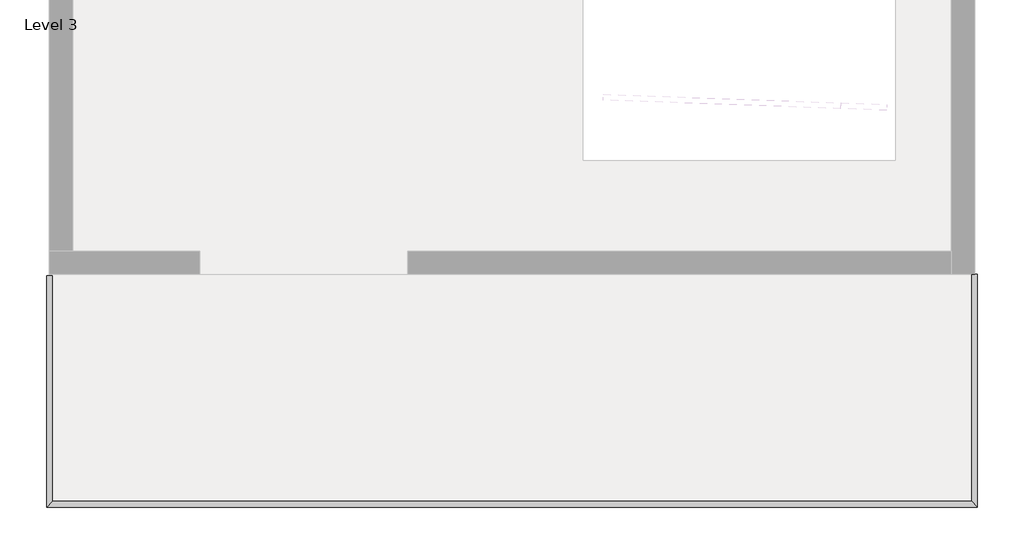
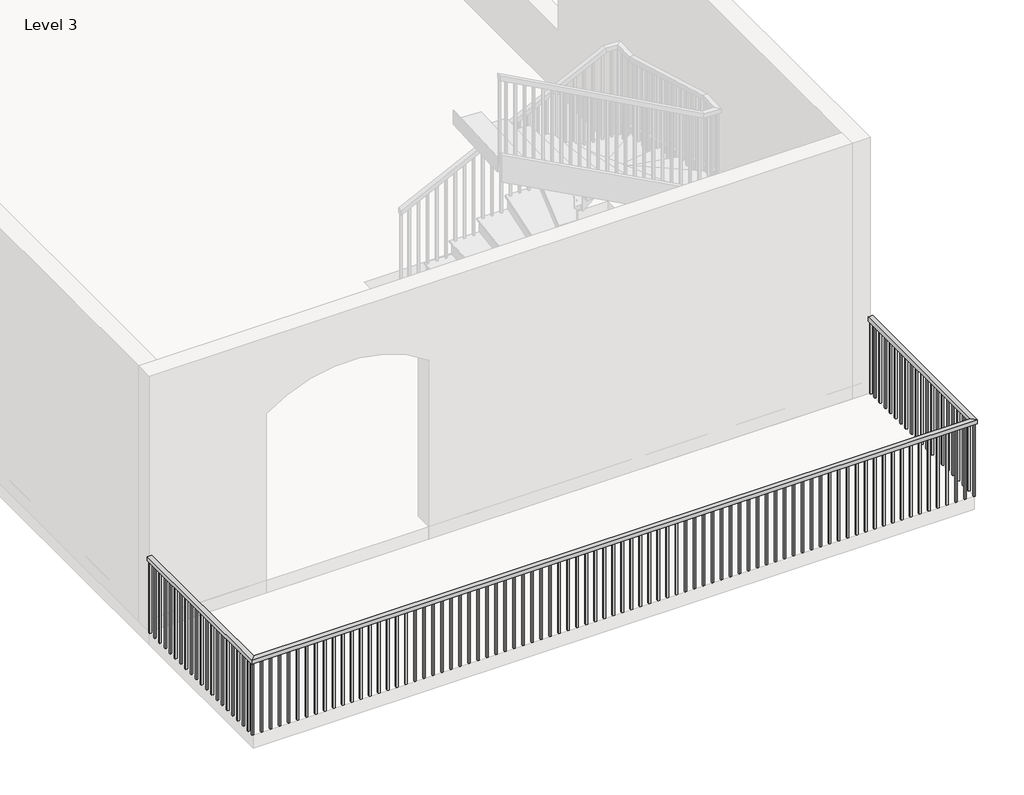
# One storey, part 2 of 3: 1 railing.
"""IFC4 building model written with IfcOpenShell, lengths in millimetres."""

from ifc_helpers import new_model, si_unit, frame, origin, place, context, project, spatial, polyline, outline, extrude, faceted_brep, element, save

model = new_model("IFC4")

# Units and contexts
model_context = context("Model", 3, world=origin())
ifc_project = project(units=[si_unit("LENGTHUNIT", "METRE", prefix="MILLI")], contexts=[model_context])

# Site, building, storey
site = spatial("IfcSite", under=ifc_project)
building = spatial("IfcBuilding", under=site)
storey = spatial("IfcBuildingStorey", under=building, Name="Level 3", Elevation=6096.0)

# Railing
placement = place(None, origin())
element("IfcRailing", 1, ObjectType="Handrail - Rectangular", at=placement, inside=storey, context=model_context, shape_type="SolidModel", body=[
    faceted_brep([(-14924.1126504, -4064.508, 7010.4), (-14924.1126504, -4064.508, 6959.6), (-14974.9126504, -4064.508, 6959.6), (-14974.9126504, -4064.508, 7010.4), (-14924.1126504, -6045.708, 7010.4), (-14924.1126504, -6045.708, 6959.6), (-14974.9126504, -6096.508, 6959.6), (-14974.9126504, -6096.508, 7010.4), (-6846.9126504, -6045.708, 7010.4), (-6846.9126504, -6045.708, 6959.6), (-6796.1126504, -6096.508, 6959.6), (-6796.1126504, -6096.508, 7010.4), (-6846.9126504, -4050.471143, 7010.4), (-6796.1126504, -4050.471143, 7010.4), (-6796.1126504, -4050.471143, 6959.6), (-6846.9126504, -4050.471143, 6959.6)], [[[0, 1, 2, 3]], [[1, 0, 4, 5]], [[2, 1, 5, 6]], [[3, 2, 6, 7]], [[0, 3, 7, 4]], [[5, 4, 8, 9]], [[6, 5, 9, 10]], [[7, 6, 10, 11]], [[4, 7, 11, 8]], [[12, 13, 14, 15]], [[9, 8, 12, 15]], [[10, 9, 15, 14]], [[11, 10, 14, 13]], [[8, 11, 13, 12]]]),
    extrude(outline(polyline([(-6811.9876504, -4150.233), (-6831.0376504, -4150.233), (-6831.0376504, -4131.183), (-6811.9876504, -4131.183), (-6811.9876504, -4150.233)])), frame((0.0, 0.0, 6096.0), z_axis=(0.0, 0.0, 1.0), x_axis=(1.0, 0.0, 0.0)), (0.0, 0.0, 1.0), 863.6),
    extrude(outline(polyline([(-6811.9876504, -4251.833), (-6831.0376504, -4251.833), (-6831.0376504, -4232.783), (-6811.9876504, -4232.783), (-6811.9876504, -4251.833)])), frame((0.0, 0.0, 6096.0), z_axis=(0.0, 0.0, 1.0), x_axis=(1.0, 0.0, 0.0)), (0.0, 0.0, 1.0), 863.6),
    extrude(outline(polyline([(-6811.9876504, -4353.433), (-6831.0376504, -4353.433), (-6831.0376504, -4334.383), (-6811.9876504, -4334.383), (-6811.9876504, -4353.433)])), frame((0.0, 0.0, 6096.0), z_axis=(0.0, 0.0, 1.0), x_axis=(1.0, 0.0, 0.0)), (0.0, 0.0, 1.0), 863.6),
    extrude(outline(polyline([(-6811.9876504, -4455.033), (-6831.0376504, -4455.033), (-6831.0376504, -4435.983), (-6811.9876504, -4435.983), (-6811.9876504, -4455.033)])), frame((0.0, 0.0, 6096.0), z_axis=(0.0, 0.0, 1.0), x_axis=(1.0, 0.0, 0.0)), (0.0, 0.0, 1.0), 863.6),
    extrude(outline(polyline([(-6811.9876504, -4556.633), (-6831.0376504, -4556.633), (-6831.0376504, -4537.583), (-6811.9876504, -4537.583), (-6811.9876504, -4556.633)])), frame((0.0, 0.0, 6096.0), z_axis=(0.0, 0.0, 1.0), x_axis=(1.0, 0.0, 0.0)), (0.0, 0.0, 1.0), 863.6),
    extrude(outline(polyline([(-6811.9876504, -4658.233), (-6831.0376504, -4658.233), (-6831.0376504, -4639.183), (-6811.9876504, -4639.183), (-6811.9876504, -4658.233)])), frame((0.0, 0.0, 6096.0), z_axis=(0.0, 0.0, 1.0), x_axis=(1.0, 0.0, 0.0)), (0.0, 0.0, 1.0), 863.6),
    extrude(outline(polyline([(-6811.9876504, -4759.833), (-6831.0376504, -4759.833), (-6831.0376504, -4740.783), (-6811.9876504, -4740.783), (-6811.9876504, -4759.833)])), frame((0.0, 0.0, 6096.0), z_axis=(0.0, 0.0, 1.0), x_axis=(1.0, 0.0, 0.0)), (0.0, 0.0, 1.0), 863.6),
    extrude(outline(polyline([(-6811.9876504, -4861.433), (-6831.0376504, -4861.433), (-6831.0376504, -4842.383), (-6811.9876504, -4842.383), (-6811.9876504, -4861.433)])), frame((0.0, 0.0, 6096.0), z_axis=(0.0, 0.0, 1.0), x_axis=(1.0, 0.0, 0.0)), (0.0, 0.0, 1.0), 863.6),
    extrude(outline(polyline([(-6811.9876504, -4963.033), (-6831.0376504, -4963.033), (-6831.0376504, -4943.983), (-6811.9876504, -4943.983), (-6811.9876504, -4963.033)])), frame((0.0, 0.0, 6096.0), z_axis=(0.0, 0.0, 1.0), x_axis=(1.0, 0.0, 0.0)), (0.0, 0.0, 1.0), 863.6),
    extrude(outline(polyline([(-6811.9876504, -5064.633), (-6831.0376504, -5064.633), (-6831.0376504, -5045.583), (-6811.9876504, -5045.583), (-6811.9876504, -5064.633)])), frame((0.0, 0.0, 6096.0), z_axis=(0.0, 0.0, 1.0), x_axis=(1.0, 0.0, 0.0)), (0.0, 0.0, 1.0), 863.6),
    extrude(outline(polyline([(-6811.9876504, -5166.233), (-6831.0376504, -5166.233), (-6831.0376504, -5147.183), (-6811.9876504, -5147.183), (-6811.9876504, -5166.233)])), frame((0.0, 0.0, 6096.0), z_axis=(0.0, 0.0, 1.0), x_axis=(1.0, 0.0, 0.0)), (0.0, 0.0, 1.0), 863.6),
    extrude(outline(polyline([(-6811.9876504, -5267.833), (-6831.0376504, -5267.833), (-6831.0376504, -5248.783), (-6811.9876504, -5248.783), (-6811.9876504, -5267.833)])), frame((0.0, 0.0, 6096.0), z_axis=(0.0, 0.0, 1.0), x_axis=(1.0, 0.0, 0.0)), (0.0, 0.0, 1.0), 863.6),
    extrude(outline(polyline([(-6811.9876504, -5369.433), (-6831.0376504, -5369.433), (-6831.0376504, -5350.383), (-6811.9876504, -5350.383), (-6811.9876504, -5369.433)])), frame((0.0, 0.0, 6096.0), z_axis=(0.0, 0.0, 1.0), x_axis=(1.0, 0.0, 0.0)), (0.0, 0.0, 1.0), 863.6),
    extrude(outline(polyline([(-6811.9876504, -5471.033), (-6831.0376504, -5471.033), (-6831.0376504, -5451.983), (-6811.9876504, -5451.983), (-6811.9876504, -5471.033)])), frame((0.0, 0.0, 6096.0), z_axis=(0.0, 0.0, 1.0), x_axis=(1.0, 0.0, 0.0)), (0.0, 0.0, 1.0), 863.6),
    extrude(outline(polyline([(-6811.9876504, -5572.633), (-6831.0376504, -5572.633), (-6831.0376504, -5553.583), (-6811.9876504, -5553.583), (-6811.9876504, -5572.633)])), frame((0.0, 0.0, 6096.0), z_axis=(0.0, 0.0, 1.0), x_axis=(1.0, 0.0, 0.0)), (0.0, 0.0, 1.0), 863.6),
    extrude(outline(polyline([(-6811.9876504, -5674.233), (-6831.0376504, -5674.233), (-6831.0376504, -5655.183), (-6811.9876504, -5655.183), (-6811.9876504, -5674.233)])), frame((0.0, 0.0, 6096.0), z_axis=(0.0, 0.0, 1.0), x_axis=(1.0, 0.0, 0.0)), (0.0, 0.0, 1.0), 863.6),
    extrude(outline(polyline([(-6811.9876504, -5775.833), (-6831.0376504, -5775.833), (-6831.0376504, -5756.783), (-6811.9876504, -5756.783), (-6811.9876504, -5775.833)])), frame((0.0, 0.0, 6096.0), z_axis=(0.0, 0.0, 1.0), x_axis=(1.0, 0.0, 0.0)), (0.0, 0.0, 1.0), 863.6),
    extrude(outline(polyline([(-6811.9876504, -5877.433), (-6831.0376504, -5877.433), (-6831.0376504, -5858.383), (-6811.9876504, -5858.383), (-6811.9876504, -5877.433)])), frame((0.0, 0.0, 6096.0), z_axis=(0.0, 0.0, 1.0), x_axis=(1.0, 0.0, 0.0)), (0.0, 0.0, 1.0), 863.6),
    extrude(outline(polyline([(-6811.9876504, -5979.033), (-6831.0376504, -5979.033), (-6831.0376504, -5959.983), (-6811.9876504, -5959.983), (-6811.9876504, -5979.033)])), frame((0.0, 0.0, 6096.0), z_axis=(0.0, 0.0, 1.0), x_axis=(1.0, 0.0, 0.0)), (0.0, 0.0, 1.0), 863.6),
    extrude(outline(polyline([(-6932.6376504, -6080.633), (-6932.6376504, -6061.583), (-6913.5876504, -6061.583), (-6913.5876504, -6080.633), (-6932.6376504, -6080.633)])), frame((0.0, 0.0, 6096.0), z_axis=(0.0, 0.0, 1.0), x_axis=(1.0, 0.0, 0.0)), (0.0, 0.0, 1.0), 863.6),
    extrude(outline(polyline([(-7034.2376504, -6080.633), (-7034.2376504, -6061.583), (-7015.1876504, -6061.583), (-7015.1876504, -6080.633), (-7034.2376504, -6080.633)])), frame((0.0, 0.0, 6096.0), z_axis=(0.0, 0.0, 1.0), x_axis=(1.0, 0.0, 0.0)), (0.0, 0.0, 1.0), 863.6),
    extrude(outline(polyline([(-7135.8376504, -6080.633), (-7135.8376504, -6061.583), (-7116.7876504, -6061.583), (-7116.7876504, -6080.633), (-7135.8376504, -6080.633)])), frame((0.0, 0.0, 6096.0), z_axis=(0.0, 0.0, 1.0), x_axis=(1.0, 0.0, 0.0)), (0.0, 0.0, 1.0), 863.6),
    extrude(outline(polyline([(-7237.4376504, -6080.633), (-7237.4376504, -6061.583), (-7218.3876504, -6061.583), (-7218.3876504, -6080.633), (-7237.4376504, -6080.633)])), frame((0.0, 0.0, 6096.0), z_axis=(0.0, 0.0, 1.0), x_axis=(1.0, 0.0, 0.0)), (0.0, 0.0, 1.0), 863.6),
    extrude(outline(polyline([(-7339.0376504, -6080.633), (-7339.0376504, -6061.583), (-7319.9876504, -6061.583), (-7319.9876504, -6080.633), (-7339.0376504, -6080.633)])), frame((0.0, 0.0, 6096.0), z_axis=(0.0, 0.0, 1.0), x_axis=(1.0, 0.0, 0.0)), (0.0, 0.0, 1.0), 863.6),
    extrude(outline(polyline([(-7440.6376504, -6080.633), (-7440.6376504, -6061.583), (-7421.5876504, -6061.583), (-7421.5876504, -6080.633), (-7440.6376504, -6080.633)])), frame((0.0, 0.0, 6096.0), z_axis=(0.0, 0.0, 1.0), x_axis=(1.0, 0.0, 0.0)), (0.0, 0.0, 1.0), 863.6),
    extrude(outline(polyline([(-7542.2376504, -6080.633), (-7542.2376504, -6061.583), (-7523.1876504, -6061.583), (-7523.1876504, -6080.633), (-7542.2376504, -6080.633)])), frame((0.0, 0.0, 6096.0), z_axis=(0.0, 0.0, 1.0), x_axis=(1.0, 0.0, 0.0)), (0.0, 0.0, 1.0), 863.6),
    extrude(outline(polyline([(-7643.8376504, -6080.633), (-7643.8376504, -6061.583), (-7624.7876504, -6061.583), (-7624.7876504, -6080.633), (-7643.8376504, -6080.633)])), frame((0.0, 0.0, 6096.0), z_axis=(0.0, 0.0, 1.0), x_axis=(1.0, 0.0, 0.0)), (0.0, 0.0, 1.0), 863.6),
    extrude(outline(polyline([(-7745.4376504, -6080.633), (-7745.4376504, -6061.583), (-7726.3876504, -6061.583), (-7726.3876504, -6080.633), (-7745.4376504, -6080.633)])), frame((0.0, 0.0, 6096.0), z_axis=(0.0, 0.0, 1.0), x_axis=(1.0, 0.0, 0.0)), (0.0, 0.0, 1.0), 863.6),
    extrude(outline(polyline([(-7847.0376504, -6080.633), (-7847.0376504, -6061.583), (-7827.9876504, -6061.583), (-7827.9876504, -6080.633), (-7847.0376504, -6080.633)])), frame((0.0, 0.0, 6096.0), z_axis=(0.0, 0.0, 1.0), x_axis=(1.0, 0.0, 0.0)), (0.0, 0.0, 1.0), 863.6),
    extrude(outline(polyline([(-7948.6376504, -6080.633), (-7948.6376504, -6061.583), (-7929.5876504, -6061.583), (-7929.5876504, -6080.633), (-7948.6376504, -6080.633)])), frame((0.0, 0.0, 6096.0), z_axis=(0.0, 0.0, 1.0), x_axis=(1.0, 0.0, 0.0)), (0.0, 0.0, 1.0), 863.6),
    extrude(outline(polyline([(-8050.2376504, -6080.633), (-8050.2376504, -6061.583), (-8031.1876504, -6061.583), (-8031.1876504, -6080.633), (-8050.2376504, -6080.633)])), frame((0.0, 0.0, 6096.0), z_axis=(0.0, 0.0, 1.0), x_axis=(1.0, 0.0, 0.0)), (0.0, 0.0, 1.0), 863.6),
    extrude(outline(polyline([(-8151.8376504, -6080.633), (-8151.8376504, -6061.583), (-8132.7876504, -6061.583), (-8132.7876504, -6080.633), (-8151.8376504, -6080.633)])), frame((0.0, 0.0, 6096.0), z_axis=(0.0, 0.0, 1.0), x_axis=(1.0, 0.0, 0.0)), (0.0, 0.0, 1.0), 863.6),
    extrude(outline(polyline([(-8253.4376504, -6080.633), (-8253.4376504, -6061.583), (-8234.3876504, -6061.583), (-8234.3876504, -6080.633), (-8253.4376504, -6080.633)])), frame((0.0, 0.0, 6096.0), z_axis=(0.0, 0.0, 1.0), x_axis=(1.0, 0.0, 0.0)), (0.0, 0.0, 1.0), 863.6),
    extrude(outline(polyline([(-8355.0376504, -6080.633), (-8355.0376504, -6061.583), (-8335.9876504, -6061.583), (-8335.9876504, -6080.633), (-8355.0376504, -6080.633)])), frame((0.0, 0.0, 6096.0), z_axis=(0.0, 0.0, 1.0), x_axis=(1.0, 0.0, 0.0)), (0.0, 0.0, 1.0), 863.6),
    extrude(outline(polyline([(-8456.6376504, -6080.633), (-8456.6376504, -6061.583), (-8437.5876504, -6061.583), (-8437.5876504, -6080.633), (-8456.6376504, -6080.633)])), frame((0.0, 0.0, 6096.0), z_axis=(0.0, 0.0, 1.0), x_axis=(1.0, 0.0, 0.0)), (0.0, 0.0, 1.0), 863.6),
    extrude(outline(polyline([(-8558.2376504, -6080.633), (-8558.2376504, -6061.583), (-8539.1876504, -6061.583), (-8539.1876504, -6080.633), (-8558.2376504, -6080.633)])), frame((0.0, 0.0, 6096.0), z_axis=(0.0, 0.0, 1.0), x_axis=(1.0, 0.0, 0.0)), (0.0, 0.0, 1.0), 863.6),
    extrude(outline(polyline([(-8659.8376504, -6080.633), (-8659.8376504, -6061.583), (-8640.7876504, -6061.583), (-8640.7876504, -6080.633), (-8659.8376504, -6080.633)])), frame((0.0, 0.0, 6096.0), z_axis=(0.0, 0.0, 1.0), x_axis=(1.0, 0.0, 0.0)), (0.0, 0.0, 1.0), 863.6),
    extrude(outline(polyline([(-8761.4376504, -6080.633), (-8761.4376504, -6061.583), (-8742.3876504, -6061.583), (-8742.3876504, -6080.633), (-8761.4376504, -6080.633)])), frame((0.0, 0.0, 6096.0), z_axis=(0.0, 0.0, 1.0), x_axis=(1.0, 0.0, 0.0)), (0.0, 0.0, 1.0), 863.6),
    extrude(outline(polyline([(-8863.0376504, -6080.633), (-8863.0376504, -6061.583), (-8843.9876504, -6061.583), (-8843.9876504, -6080.633), (-8863.0376504, -6080.633)])), frame((0.0, 0.0, 6096.0), z_axis=(0.0, 0.0, 1.0), x_axis=(1.0, 0.0, 0.0)), (0.0, 0.0, 1.0), 863.6),
    extrude(outline(polyline([(-8964.6376504, -6080.633), (-8964.6376504, -6061.583), (-8945.5876504, -6061.583), (-8945.5876504, -6080.633), (-8964.6376504, -6080.633)])), frame((0.0, 0.0, 6096.0), z_axis=(0.0, 0.0, 1.0), x_axis=(1.0, 0.0, 0.0)), (0.0, 0.0, 1.0), 863.6),
    extrude(outline(polyline([(-9066.2376504, -6080.633), (-9066.2376504, -6061.583), (-9047.1876504, -6061.583), (-9047.1876504, -6080.633), (-9066.2376504, -6080.633)])), frame((0.0, 0.0, 6096.0), z_axis=(0.0, 0.0, 1.0), x_axis=(1.0, 0.0, 0.0)), (0.0, 0.0, 1.0), 863.6),
    extrude(outline(polyline([(-9167.8376504, -6080.633), (-9167.8376504, -6061.583), (-9148.7876504, -6061.583), (-9148.7876504, -6080.633), (-9167.8376504, -6080.633)])), frame((0.0, 0.0, 6096.0), z_axis=(0.0, 0.0, 1.0), x_axis=(1.0, 0.0, 0.0)), (0.0, 0.0, 1.0), 863.6),
    extrude(outline(polyline([(-9269.4376504, -6080.633), (-9269.4376504, -6061.583), (-9250.3876504, -6061.583), (-9250.3876504, -6080.633), (-9269.4376504, -6080.633)])), frame((0.0, 0.0, 6096.0), z_axis=(0.0, 0.0, 1.0), x_axis=(1.0, 0.0, 0.0)), (0.0, 0.0, 1.0), 863.6),
    extrude(outline(polyline([(-9371.0376504, -6080.633), (-9371.0376504, -6061.583), (-9351.9876504, -6061.583), (-9351.9876504, -6080.633), (-9371.0376504, -6080.633)])), frame((0.0, 0.0, 6096.0), z_axis=(0.0, 0.0, 1.0), x_axis=(1.0, 0.0, 0.0)), (0.0, 0.0, 1.0), 863.6),
    extrude(outline(polyline([(-9472.6376504, -6080.633), (-9472.6376504, -6061.583), (-9453.5876504, -6061.583), (-9453.5876504, -6080.633), (-9472.6376504, -6080.633)])), frame((0.0, 0.0, 6096.0), z_axis=(0.0, 0.0, 1.0), x_axis=(1.0, 0.0, 0.0)), (0.0, 0.0, 1.0), 863.6),
    extrude(outline(polyline([(-9574.2376504, -6080.633), (-9574.2376504, -6061.583), (-9555.1876504, -6061.583), (-9555.1876504, -6080.633), (-9574.2376504, -6080.633)])), frame((0.0, 0.0, 6096.0), z_axis=(0.0, 0.0, 1.0), x_axis=(1.0, 0.0, 0.0)), (0.0, 0.0, 1.0), 863.6),
    extrude(outline(polyline([(-9675.8376504, -6080.633), (-9675.8376504, -6061.583), (-9656.7876504, -6061.583), (-9656.7876504, -6080.633), (-9675.8376504, -6080.633)])), frame((0.0, 0.0, 6096.0), z_axis=(0.0, 0.0, 1.0), x_axis=(1.0, 0.0, 0.0)), (0.0, 0.0, 1.0), 863.6),
    extrude(outline(polyline([(-9777.4376504, -6080.633), (-9777.4376504, -6061.583), (-9758.3876504, -6061.583), (-9758.3876504, -6080.633), (-9777.4376504, -6080.633)])), frame((0.0, 0.0, 6096.0), z_axis=(0.0, 0.0, 1.0), x_axis=(1.0, 0.0, 0.0)), (0.0, 0.0, 1.0), 863.6),
    extrude(outline(polyline([(-9879.0376504, -6080.633), (-9879.0376504, -6061.583), (-9859.9876504, -6061.583), (-9859.9876504, -6080.633), (-9879.0376504, -6080.633)])), frame((0.0, 0.0, 6096.0), z_axis=(0.0, 0.0, 1.0), x_axis=(1.0, 0.0, 0.0)), (0.0, 0.0, 1.0), 863.6),
    extrude(outline(polyline([(-9980.6376504, -6080.633), (-9980.6376504, -6061.583), (-9961.5876504, -6061.583), (-9961.5876504, -6080.633), (-9980.6376504, -6080.633)])), frame((0.0, 0.0, 6096.0), z_axis=(0.0, 0.0, 1.0), x_axis=(1.0, 0.0, 0.0)), (0.0, 0.0, 1.0), 863.6),
    extrude(outline(polyline([(-10082.2376504, -6080.633), (-10082.2376504, -6061.583), (-10063.1876504, -6061.583), (-10063.1876504, -6080.633), (-10082.2376504, -6080.633)])), frame((0.0, 0.0, 6096.0), z_axis=(0.0, 0.0, 1.0), x_axis=(1.0, 0.0, 0.0)), (0.0, 0.0, 1.0), 863.6),
    extrude(outline(polyline([(-10183.8376504, -6080.633), (-10183.8376504, -6061.583), (-10164.7876504, -6061.583), (-10164.7876504, -6080.633), (-10183.8376504, -6080.633)])), frame((0.0, 0.0, 6096.0), z_axis=(0.0, 0.0, 1.0), x_axis=(1.0, 0.0, 0.0)), (0.0, 0.0, 1.0), 863.6),
    extrude(outline(polyline([(-10285.4376504, -6080.633), (-10285.4376504, -6061.583), (-10266.3876504, -6061.583), (-10266.3876504, -6080.633), (-10285.4376504, -6080.633)])), frame((0.0, 0.0, 6096.0), z_axis=(0.0, 0.0, 1.0), x_axis=(1.0, 0.0, 0.0)), (0.0, 0.0, 1.0), 863.6),
    extrude(outline(polyline([(-10387.0376504, -6080.633), (-10387.0376504, -6061.583), (-10367.9876504, -6061.583), (-10367.9876504, -6080.633), (-10387.0376504, -6080.633)])), frame((0.0, 0.0, 6096.0), z_axis=(0.0, 0.0, 1.0), x_axis=(1.0, 0.0, 0.0)), (0.0, 0.0, 1.0), 863.6),
    extrude(outline(polyline([(-10488.6376504, -6080.633), (-10488.6376504, -6061.583), (-10469.5876504, -6061.583), (-10469.5876504, -6080.633), (-10488.6376504, -6080.633)])), frame((0.0, 0.0, 6096.0), z_axis=(0.0, 0.0, 1.0), x_axis=(1.0, 0.0, 0.0)), (0.0, 0.0, 1.0), 863.6),
    extrude(outline(polyline([(-10590.2376504, -6080.633), (-10590.2376504, -6061.583), (-10571.1876504, -6061.583), (-10571.1876504, -6080.633), (-10590.2376504, -6080.633)])), frame((0.0, 0.0, 6096.0), z_axis=(0.0, 0.0, 1.0), x_axis=(1.0, 0.0, 0.0)), (0.0, 0.0, 1.0), 863.6),
    extrude(outline(polyline([(-10691.8376504, -6080.633), (-10691.8376504, -6061.583), (-10672.7876504, -6061.583), (-10672.7876504, -6080.633), (-10691.8376504, -6080.633)])), frame((0.0, 0.0, 6096.0), z_axis=(0.0, 0.0, 1.0), x_axis=(1.0, 0.0, 0.0)), (0.0, 0.0, 1.0), 863.6),
    extrude(outline(polyline([(-10793.4376504, -6080.633), (-10793.4376504, -6061.583), (-10774.3876504, -6061.583), (-10774.3876504, -6080.633), (-10793.4376504, -6080.633)])), frame((0.0, 0.0, 6096.0), z_axis=(0.0, 0.0, 1.0), x_axis=(1.0, 0.0, 0.0)), (0.0, 0.0, 1.0), 863.6),
    extrude(outline(polyline([(-10895.0376504, -6080.633), (-10895.0376504, -6061.583), (-10875.9876504, -6061.583), (-10875.9876504, -6080.633), (-10895.0376504, -6080.633)])), frame((0.0, 0.0, 6096.0), z_axis=(0.0, 0.0, 1.0), x_axis=(1.0, 0.0, 0.0)), (0.0, 0.0, 1.0), 863.6),
    extrude(outline(polyline([(-10996.6376504, -6080.633), (-10996.6376504, -6061.583), (-10977.5876504, -6061.583), (-10977.5876504, -6080.633), (-10996.6376504, -6080.633)])), frame((0.0, 0.0, 6096.0), z_axis=(0.0, 0.0, 1.0), x_axis=(1.0, 0.0, 0.0)), (0.0, 0.0, 1.0), 863.6),
    extrude(outline(polyline([(-11098.2376504, -6080.633), (-11098.2376504, -6061.583), (-11079.1876504, -6061.583), (-11079.1876504, -6080.633), (-11098.2376504, -6080.633)])), frame((0.0, 0.0, 6096.0), z_axis=(0.0, 0.0, 1.0), x_axis=(1.0, 0.0, 0.0)), (0.0, 0.0, 1.0), 863.6),
    extrude(outline(polyline([(-11199.8376504, -6080.633), (-11199.8376504, -6061.583), (-11180.7876504, -6061.583), (-11180.7876504, -6080.633), (-11199.8376504, -6080.633)])), frame((0.0, 0.0, 6096.0), z_axis=(0.0, 0.0, 1.0), x_axis=(1.0, 0.0, 0.0)), (0.0, 0.0, 1.0), 863.6),
    extrude(outline(polyline([(-11301.4376504, -6080.633), (-11301.4376504, -6061.583), (-11282.3876504, -6061.583), (-11282.3876504, -6080.633), (-11301.4376504, -6080.633)])), frame((0.0, 0.0, 6096.0), z_axis=(0.0, 0.0, 1.0), x_axis=(1.0, 0.0, 0.0)), (0.0, 0.0, 1.0), 863.6),
    extrude(outline(polyline([(-11403.0376504, -6080.633), (-11403.0376504, -6061.583), (-11383.9876504, -6061.583), (-11383.9876504, -6080.633), (-11403.0376504, -6080.633)])), frame((0.0, 0.0, 6096.0), z_axis=(0.0, 0.0, 1.0), x_axis=(1.0, 0.0, 0.0)), (0.0, 0.0, 1.0), 863.6),
    extrude(outline(polyline([(-11504.6376504, -6080.633), (-11504.6376504, -6061.583), (-11485.5876504, -6061.583), (-11485.5876504, -6080.633), (-11504.6376504, -6080.633)])), frame((0.0, 0.0, 6096.0), z_axis=(0.0, 0.0, 1.0), x_axis=(1.0, 0.0, 0.0)), (0.0, 0.0, 1.0), 863.6),
    extrude(outline(polyline([(-11606.2376504, -6080.633), (-11606.2376504, -6061.583), (-11587.1876504, -6061.583), (-11587.1876504, -6080.633), (-11606.2376504, -6080.633)])), frame((0.0, 0.0, 6096.0), z_axis=(0.0, 0.0, 1.0), x_axis=(1.0, 0.0, 0.0)), (0.0, 0.0, 1.0), 863.6),
    extrude(outline(polyline([(-11707.8376504, -6080.633), (-11707.8376504, -6061.583), (-11688.7876504, -6061.583), (-11688.7876504, -6080.633), (-11707.8376504, -6080.633)])), frame((0.0, 0.0, 6096.0), z_axis=(0.0, 0.0, 1.0), x_axis=(1.0, 0.0, 0.0)), (0.0, 0.0, 1.0), 863.6),
    extrude(outline(polyline([(-11809.4376504, -6080.633), (-11809.4376504, -6061.583), (-11790.3876504, -6061.583), (-11790.3876504, -6080.633), (-11809.4376504, -6080.633)])), frame((0.0, 0.0, 6096.0), z_axis=(0.0, 0.0, 1.0), x_axis=(1.0, 0.0, 0.0)), (0.0, 0.0, 1.0), 863.6),
    extrude(outline(polyline([(-11911.0376504, -6080.633), (-11911.0376504, -6061.583), (-11891.9876504, -6061.583), (-11891.9876504, -6080.633), (-11911.0376504, -6080.633)])), frame((0.0, 0.0, 6096.0), z_axis=(0.0, 0.0, 1.0), x_axis=(1.0, 0.0, 0.0)), (0.0, 0.0, 1.0), 863.6),
    extrude(outline(polyline([(-12012.6376504, -6080.633), (-12012.6376504, -6061.583), (-11993.5876504, -6061.583), (-11993.5876504, -6080.633), (-12012.6376504, -6080.633)])), frame((0.0, 0.0, 6096.0), z_axis=(0.0, 0.0, 1.0), x_axis=(1.0, 0.0, 0.0)), (0.0, 0.0, 1.0), 863.6),
    extrude(outline(polyline([(-12114.2376504, -6080.633), (-12114.2376504, -6061.583), (-12095.1876504, -6061.583), (-12095.1876504, -6080.633), (-12114.2376504, -6080.633)])), frame((0.0, 0.0, 6096.0), z_axis=(0.0, 0.0, 1.0), x_axis=(1.0, 0.0, 0.0)), (0.0, 0.0, 1.0), 863.6),
    extrude(outline(polyline([(-12215.8376504, -6080.633), (-12215.8376504, -6061.583), (-12196.7876504, -6061.583), (-12196.7876504, -6080.633), (-12215.8376504, -6080.633)])), frame((0.0, 0.0, 6096.0), z_axis=(0.0, 0.0, 1.0), x_axis=(1.0, 0.0, 0.0)), (0.0, 0.0, 1.0), 863.6),
    extrude(outline(polyline([(-12317.4376504, -6080.633), (-12317.4376504, -6061.583), (-12298.3876504, -6061.583), (-12298.3876504, -6080.633), (-12317.4376504, -6080.633)])), frame((0.0, 0.0, 6096.0), z_axis=(0.0, 0.0, 1.0), x_axis=(1.0, 0.0, 0.0)), (0.0, 0.0, 1.0), 863.6),
    extrude(outline(polyline([(-12419.0376504, -6080.633), (-12419.0376504, -6061.583), (-12399.9876504, -6061.583), (-12399.9876504, -6080.633), (-12419.0376504, -6080.633)])), frame((0.0, 0.0, 6096.0), z_axis=(0.0, 0.0, 1.0), x_axis=(1.0, 0.0, 0.0)), (0.0, 0.0, 1.0), 863.6),
    extrude(outline(polyline([(-12520.6376504, -6080.633), (-12520.6376504, -6061.583), (-12501.5876504, -6061.583), (-12501.5876504, -6080.633), (-12520.6376504, -6080.633)])), frame((0.0, 0.0, 6096.0), z_axis=(0.0, 0.0, 1.0), x_axis=(1.0, 0.0, 0.0)), (0.0, 0.0, 1.0), 863.6),
    extrude(outline(polyline([(-12622.2376504, -6080.633), (-12622.2376504, -6061.583), (-12603.1876504, -6061.583), (-12603.1876504, -6080.633), (-12622.2376504, -6080.633)])), frame((0.0, 0.0, 6096.0), z_axis=(0.0, 0.0, 1.0), x_axis=(1.0, 0.0, 0.0)), (0.0, 0.0, 1.0), 863.6),
    extrude(outline(polyline([(-12723.8376504, -6080.633), (-12723.8376504, -6061.583), (-12704.7876504, -6061.583), (-12704.7876504, -6080.633), (-12723.8376504, -6080.633)])), frame((0.0, 0.0, 6096.0), z_axis=(0.0, 0.0, 1.0), x_axis=(1.0, 0.0, 0.0)), (0.0, 0.0, 1.0), 863.6),
    extrude(outline(polyline([(-12825.4376504, -6080.633), (-12825.4376504, -6061.583), (-12806.3876504, -6061.583), (-12806.3876504, -6080.633), (-12825.4376504, -6080.633)])), frame((0.0, 0.0, 6096.0), z_axis=(0.0, 0.0, 1.0), x_axis=(1.0, 0.0, 0.0)), (0.0, 0.0, 1.0), 863.6),
    extrude(outline(polyline([(-12927.0376504, -6080.633), (-12927.0376504, -6061.583), (-12907.9876504, -6061.583), (-12907.9876504, -6080.633), (-12927.0376504, -6080.633)])), frame((0.0, 0.0, 6096.0), z_axis=(0.0, 0.0, 1.0), x_axis=(1.0, 0.0, 0.0)), (0.0, 0.0, 1.0), 863.6),
    extrude(outline(polyline([(-13028.6376504, -6080.633), (-13028.6376504, -6061.583), (-13009.5876504, -6061.583), (-13009.5876504, -6080.633), (-13028.6376504, -6080.633)])), frame((0.0, 0.0, 6096.0), z_axis=(0.0, 0.0, 1.0), x_axis=(1.0, 0.0, 0.0)), (0.0, 0.0, 1.0), 863.6),
    extrude(outline(polyline([(-13130.2376504, -6080.633), (-13130.2376504, -6061.583), (-13111.1876504, -6061.583), (-13111.1876504, -6080.633), (-13130.2376504, -6080.633)])), frame((0.0, 0.0, 6096.0), z_axis=(0.0, 0.0, 1.0), x_axis=(1.0, 0.0, 0.0)), (0.0, 0.0, 1.0), 863.6),
    extrude(outline(polyline([(-13231.8376504, -6080.633), (-13231.8376504, -6061.583), (-13212.7876504, -6061.583), (-13212.7876504, -6080.633), (-13231.8376504, -6080.633)])), frame((0.0, 0.0, 6096.0), z_axis=(0.0, 0.0, 1.0), x_axis=(1.0, 0.0, 0.0)), (0.0, 0.0, 1.0), 863.6),
    extrude(outline(polyline([(-13333.4376504, -6080.633), (-13333.4376504, -6061.583), (-13314.3876504, -6061.583), (-13314.3876504, -6080.633), (-13333.4376504, -6080.633)])), frame((0.0, 0.0, 6096.0), z_axis=(0.0, 0.0, 1.0), x_axis=(1.0, 0.0, 0.0)), (0.0, 0.0, 1.0), 863.6),
    extrude(outline(polyline([(-13435.0376504, -6080.633), (-13435.0376504, -6061.583), (-13415.9876504, -6061.583), (-13415.9876504, -6080.633), (-13435.0376504, -6080.633)])), frame((0.0, 0.0, 6096.0), z_axis=(0.0, 0.0, 1.0), x_axis=(1.0, 0.0, 0.0)), (0.0, 0.0, 1.0), 863.6),
    extrude(outline(polyline([(-13536.6376504, -6080.633), (-13536.6376504, -6061.583), (-13517.5876504, -6061.583), (-13517.5876504, -6080.633), (-13536.6376504, -6080.633)])), frame((0.0, 0.0, 6096.0), z_axis=(0.0, 0.0, 1.0), x_axis=(1.0, 0.0, 0.0)), (0.0, 0.0, 1.0), 863.6),
    extrude(outline(polyline([(-13638.2376504, -6080.633), (-13638.2376504, -6061.583), (-13619.1876504, -6061.583), (-13619.1876504, -6080.633), (-13638.2376504, -6080.633)])), frame((0.0, 0.0, 6096.0), z_axis=(0.0, 0.0, 1.0), x_axis=(1.0, 0.0, 0.0)), (0.0, 0.0, 1.0), 863.6),
    extrude(outline(polyline([(-13739.8376504, -6080.633), (-13739.8376504, -6061.583), (-13720.7876504, -6061.583), (-13720.7876504, -6080.633), (-13739.8376504, -6080.633)])), frame((0.0, 0.0, 6096.0), z_axis=(0.0, 0.0, 1.0), x_axis=(1.0, 0.0, 0.0)), (0.0, 0.0, 1.0), 863.6),
    extrude(outline(polyline([(-13841.4376504, -6080.633), (-13841.4376504, -6061.583), (-13822.3876504, -6061.583), (-13822.3876504, -6080.633), (-13841.4376504, -6080.633)])), frame((0.0, 0.0, 6096.0), z_axis=(0.0, 0.0, 1.0), x_axis=(1.0, 0.0, 0.0)), (0.0, 0.0, 1.0), 863.6),
    extrude(outline(polyline([(-13943.0376504, -6080.633), (-13943.0376504, -6061.583), (-13923.9876504, -6061.583), (-13923.9876504, -6080.633), (-13943.0376504, -6080.633)])), frame((0.0, 0.0, 6096.0), z_axis=(0.0, 0.0, 1.0), x_axis=(1.0, 0.0, 0.0)), (0.0, 0.0, 1.0), 863.6),
    extrude(outline(polyline([(-14044.6376504, -6080.633), (-14044.6376504, -6061.583), (-14025.5876504, -6061.583), (-14025.5876504, -6080.633), (-14044.6376504, -6080.633)])), frame((0.0, 0.0, 6096.0), z_axis=(0.0, 0.0, 1.0), x_axis=(1.0, 0.0, 0.0)), (0.0, 0.0, 1.0), 863.6),
    extrude(outline(polyline([(-14146.2376504, -6080.633), (-14146.2376504, -6061.583), (-14127.1876504, -6061.583), (-14127.1876504, -6080.633), (-14146.2376504, -6080.633)])), frame((0.0, 0.0, 6096.0), z_axis=(0.0, 0.0, 1.0), x_axis=(1.0, 0.0, 0.0)), (0.0, 0.0, 1.0), 863.6),
    extrude(outline(polyline([(-14247.8376504, -6080.633), (-14247.8376504, -6061.583), (-14228.7876504, -6061.583), (-14228.7876504, -6080.633), (-14247.8376504, -6080.633)])), frame((0.0, 0.0, 6096.0), z_axis=(0.0, 0.0, 1.0), x_axis=(1.0, 0.0, 0.0)), (0.0, 0.0, 1.0), 863.6),
    extrude(outline(polyline([(-14349.4376504, -6080.633), (-14349.4376504, -6061.583), (-14330.3876504, -6061.583), (-14330.3876504, -6080.633), (-14349.4376504, -6080.633)])), frame((0.0, 0.0, 6096.0), z_axis=(0.0, 0.0, 1.0), x_axis=(1.0, 0.0, 0.0)), (0.0, 0.0, 1.0), 863.6),
    extrude(outline(polyline([(-14451.0376504, -6080.633), (-14451.0376504, -6061.583), (-14431.9876504, -6061.583), (-14431.9876504, -6080.633), (-14451.0376504, -6080.633)])), frame((0.0, 0.0, 6096.0), z_axis=(0.0, 0.0, 1.0), x_axis=(1.0, 0.0, 0.0)), (0.0, 0.0, 1.0), 863.6),
    extrude(outline(polyline([(-14552.6376504, -6080.633), (-14552.6376504, -6061.583), (-14533.5876504, -6061.583), (-14533.5876504, -6080.633), (-14552.6376504, -6080.633)])), frame((0.0, 0.0, 6096.0), z_axis=(0.0, 0.0, 1.0), x_axis=(1.0, 0.0, 0.0)), (0.0, 0.0, 1.0), 863.6),
    extrude(outline(polyline([(-14654.2376504, -6080.633), (-14654.2376504, -6061.583), (-14635.1876504, -6061.583), (-14635.1876504, -6080.633), (-14654.2376504, -6080.633)])), frame((0.0, 0.0, 6096.0), z_axis=(0.0, 0.0, 1.0), x_axis=(1.0, 0.0, 0.0)), (0.0, 0.0, 1.0), 863.6),
    extrude(outline(polyline([(-14755.8376504, -6080.633), (-14755.8376504, -6061.583), (-14736.7876504, -6061.583), (-14736.7876504, -6080.633), (-14755.8376504, -6080.633)])), frame((0.0, 0.0, 6096.0), z_axis=(0.0, 0.0, 1.0), x_axis=(1.0, 0.0, 0.0)), (0.0, 0.0, 1.0), 863.6),
    extrude(outline(polyline([(-14857.4376504, -6080.633), (-14857.4376504, -6061.583), (-14838.3876504, -6061.583), (-14838.3876504, -6080.633), (-14857.4376504, -6080.633)])), frame((0.0, 0.0, 6096.0), z_axis=(0.0, 0.0, 1.0), x_axis=(1.0, 0.0, 0.0)), (0.0, 0.0, 1.0), 863.6),
    extrude(outline(polyline([(-14959.0376504, -5985.383), (-14939.9876504, -5985.383), (-14939.9876504, -6004.433), (-14959.0376504, -6004.433), (-14959.0376504, -5985.383)])), frame((0.0, 0.0, 6096.0), z_axis=(0.0, 0.0, 1.0), x_axis=(1.0, 0.0, 0.0)), (0.0, 0.0, 1.0), 863.6),
    extrude(outline(polyline([(-14959.0376504, -5883.783), (-14939.9876504, -5883.783), (-14939.9876504, -5902.833), (-14959.0376504, -5902.833), (-14959.0376504, -5883.783)])), frame((0.0, 0.0, 6096.0), z_axis=(0.0, 0.0, 1.0), x_axis=(1.0, 0.0, 0.0)), (0.0, 0.0, 1.0), 863.6),
    extrude(outline(polyline([(-14959.0376504, -5782.183), (-14939.9876504, -5782.183), (-14939.9876504, -5801.233), (-14959.0376504, -5801.233), (-14959.0376504, -5782.183)])), frame((0.0, 0.0, 6096.0), z_axis=(0.0, 0.0, 1.0), x_axis=(1.0, 0.0, 0.0)), (0.0, 0.0, 1.0), 863.6),
    extrude(outline(polyline([(-14959.0376504, -5680.583), (-14939.9876504, -5680.583), (-14939.9876504, -5699.633), (-14959.0376504, -5699.633), (-14959.0376504, -5680.583)])), frame((0.0, 0.0, 6096.0), z_axis=(0.0, 0.0, 1.0), x_axis=(1.0, 0.0, 0.0)), (0.0, 0.0, 1.0), 863.6),
    extrude(outline(polyline([(-14959.0376504, -5578.983), (-14939.9876504, -5578.983), (-14939.9876504, -5598.033), (-14959.0376504, -5598.033), (-14959.0376504, -5578.983)])), frame((0.0, 0.0, 6096.0), z_axis=(0.0, 0.0, 1.0), x_axis=(1.0, 0.0, 0.0)), (0.0, 0.0, 1.0), 863.6),
    extrude(outline(polyline([(-14959.0376504, -5477.383), (-14939.9876504, -5477.383), (-14939.9876504, -5496.433), (-14959.0376504, -5496.433), (-14959.0376504, -5477.383)])), frame((0.0, 0.0, 6096.0), z_axis=(0.0, 0.0, 1.0), x_axis=(1.0, 0.0, 0.0)), (0.0, 0.0, 1.0), 863.6),
    extrude(outline(polyline([(-14959.0376504, -5375.783), (-14939.9876504, -5375.783), (-14939.9876504, -5394.833), (-14959.0376504, -5394.833), (-14959.0376504, -5375.783)])), frame((0.0, 0.0, 6096.0), z_axis=(0.0, 0.0, 1.0), x_axis=(1.0, 0.0, 0.0)), (0.0, 0.0, 1.0), 863.6),
    extrude(outline(polyline([(-14959.0376504, -5274.183), (-14939.9876504, -5274.183), (-14939.9876504, -5293.233), (-14959.0376504, -5293.233), (-14959.0376504, -5274.183)])), frame((0.0, 0.0, 6096.0), z_axis=(0.0, 0.0, 1.0), x_axis=(1.0, 0.0, 0.0)), (0.0, 0.0, 1.0), 863.6),
    extrude(outline(polyline([(-14959.0376504, -5172.583), (-14939.9876504, -5172.583), (-14939.9876504, -5191.633), (-14959.0376504, -5191.633), (-14959.0376504, -5172.583)])), frame((0.0, 0.0, 6096.0), z_axis=(0.0, 0.0, 1.0), x_axis=(1.0, 0.0, 0.0)), (0.0, 0.0, 1.0), 863.6),
    extrude(outline(polyline([(-14959.0376504, -5070.983), (-14939.9876504, -5070.983), (-14939.9876504, -5090.033), (-14959.0376504, -5090.033), (-14959.0376504, -5070.983)])), frame((0.0, 0.0, 6096.0), z_axis=(0.0, 0.0, 1.0), x_axis=(1.0, 0.0, 0.0)), (0.0, 0.0, 1.0), 863.6),
    extrude(outline(polyline([(-14959.0376504, -4969.383), (-14939.9876504, -4969.383), (-14939.9876504, -4988.433), (-14959.0376504, -4988.433), (-14959.0376504, -4969.383)])), frame((0.0, 0.0, 6096.0), z_axis=(0.0, 0.0, 1.0), x_axis=(1.0, 0.0, 0.0)), (0.0, 0.0, 1.0), 863.6),
    extrude(outline(polyline([(-14959.0376504, -4867.783), (-14939.9876504, -4867.783), (-14939.9876504, -4886.833), (-14959.0376504, -4886.833), (-14959.0376504, -4867.783)])), frame((0.0, 0.0, 6096.0), z_axis=(0.0, 0.0, 1.0), x_axis=(1.0, 0.0, 0.0)), (0.0, 0.0, 1.0), 863.6),
    extrude(outline(polyline([(-14959.0376504, -4766.183), (-14939.9876504, -4766.183), (-14939.9876504, -4785.233), (-14959.0376504, -4785.233), (-14959.0376504, -4766.183)])), frame((0.0, 0.0, 6096.0), z_axis=(0.0, 0.0, 1.0), x_axis=(1.0, 0.0, 0.0)), (0.0, 0.0, 1.0), 863.6),
    extrude(outline(polyline([(-14959.0376504, -4664.583), (-14939.9876504, -4664.583), (-14939.9876504, -4683.633), (-14959.0376504, -4683.633), (-14959.0376504, -4664.583)])), frame((0.0, 0.0, 6096.0), z_axis=(0.0, 0.0, 1.0), x_axis=(1.0, 0.0, 0.0)), (0.0, 0.0, 1.0), 863.6),
    extrude(outline(polyline([(-14959.0376504, -4562.983), (-14939.9876504, -4562.983), (-14939.9876504, -4582.033), (-14959.0376504, -4582.033), (-14959.0376504, -4562.983)])), frame((0.0, 0.0, 6096.0), z_axis=(0.0, 0.0, 1.0), x_axis=(1.0, 0.0, 0.0)), (0.0, 0.0, 1.0), 863.6),
    extrude(outline(polyline([(-14959.0376504, -4461.383), (-14939.9876504, -4461.383), (-14939.9876504, -4480.433), (-14959.0376504, -4480.433), (-14959.0376504, -4461.383)])), frame((0.0, 0.0, 6096.0), z_axis=(0.0, 0.0, 1.0), x_axis=(1.0, 0.0, 0.0)), (0.0, 0.0, 1.0), 863.6),
    extrude(outline(polyline([(-14959.0376504, -4359.783), (-14939.9876504, -4359.783), (-14939.9876504, -4378.833), (-14959.0376504, -4378.833), (-14959.0376504, -4359.783)])), frame((0.0, 0.0, 6096.0), z_axis=(0.0, 0.0, 1.0), x_axis=(1.0, 0.0, 0.0)), (0.0, 0.0, 1.0), 863.6),
    extrude(outline(polyline([(-14959.0376504, -4258.183), (-14939.9876504, -4258.183), (-14939.9876504, -4277.233), (-14959.0376504, -4277.233), (-14959.0376504, -4258.183)])), frame((0.0, 0.0, 6096.0), z_axis=(0.0, 0.0, 1.0), x_axis=(1.0, 0.0, 0.0)), (0.0, 0.0, 1.0), 863.6),
    extrude(outline(polyline([(-14959.0376504, -4156.583), (-14939.9876504, -4156.583), (-14939.9876504, -4175.633), (-14959.0376504, -4175.633), (-14959.0376504, -4156.583)])), frame((0.0, 0.0, 6096.0), z_axis=(0.0, 0.0, 1.0), x_axis=(1.0, 0.0, 0.0)), (0.0, 0.0, 1.0), 863.6),
    extrude(outline(polyline([(-6831.0376504, -6080.633), (-6831.0376504, -6061.583), (-6811.9876504, -6061.583), (-6811.9876504, -6080.633), (-6831.0376504, -6080.633)])), frame((0.0, 0.0, 6096.0), z_axis=(0.0, 0.0, 1.0), x_axis=(1.0, 0.0, 0.0)), (0.0, 0.0, 1.0), 863.6),
    extrude(outline(polyline([(-14959.0376504, -6061.583), (-14939.9876504, -6061.583), (-14939.9876504, -6080.633), (-14959.0376504, -6080.633), (-14959.0376504, -6061.583)])), frame((0.0, 0.0, 6096.0), z_axis=(0.0, 0.0, 1.0), x_axis=(1.0, 0.0, 0.0)), (0.0, 0.0, 1.0), 863.6),
    extrude(outline(polyline([(-6811.9876504, -4069.521143), (-6831.0376504, -4069.521143), (-6831.0376504, -4050.471143), (-6811.9876504, -4050.471143), (-6811.9876504, -4069.521143)])), frame((0.0, 0.0, 6096.0), z_axis=(0.0, 0.0, 1.0), x_axis=(1.0, 0.0, 0.0)), (0.0, 0.0, 1.0), 863.6),
    extrude(outline(polyline([(-14959.0376504, -4064.508), (-14939.9876504, -4064.508), (-14939.9876504, -4083.558), (-14959.0376504, -4083.558), (-14959.0376504, -4064.508)])), frame((0.0, 0.0, 6096.0), z_axis=(0.0, 0.0, 1.0), x_axis=(1.0, 0.0, 0.0)), (0.0, 0.0, 1.0), 863.6),
])

save(model, "model.ifc")

# Revit data of these elements
# Type "Handrail - Rectangular"
#   Assembly Code = "C2010400"
#   built-in parameter 1008612 = 0.0416667 (stored number, unit not read)
#   built-in parameter 1008611 = 0.0416667 (stored number, unit not read)
#   built-in parameter 1008609 = 0.333333 (stored number, unit not read)
#   built-in parameter 1008604 = 0.166667 (stored number, unit not read)
#   built-in parameter 1008603 = 0.166667 (stored number, unit not read)
#   Railing Height = 3' - 0"
#   built-in parameter 1008630 = 2
#   built-in parameter 1008610 = 2
#   built-in parameter 1008618 = Baluster - Square : 3/4"
# Element 1 (IfcRailing, "Handrail - Rectangular")
#   Phase Created = New Construction
